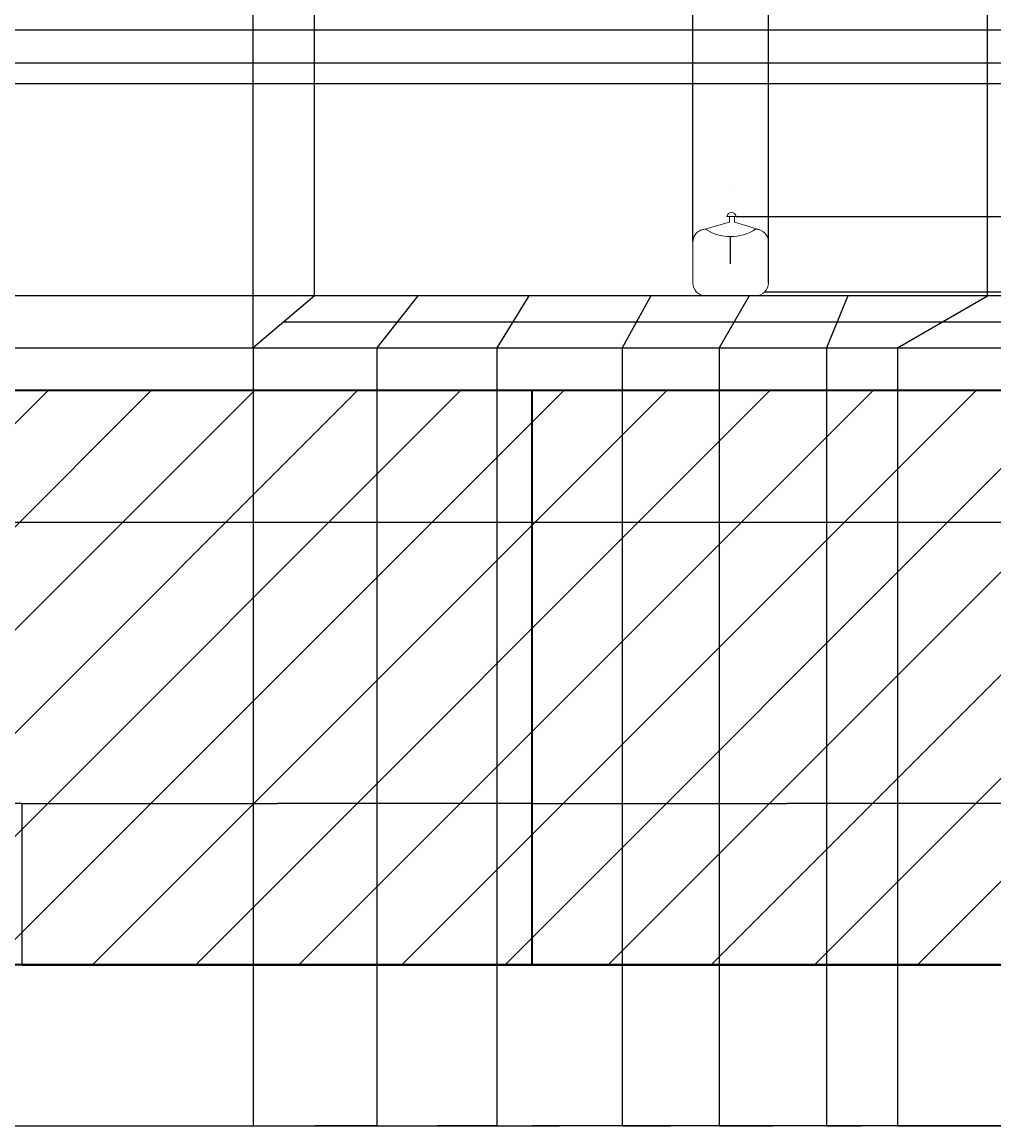
# Model space of a CAD drawing. Units: millimetres. Extents: x 2212 to 7718, y 1114 to 4219.
# Tile 2 of 5: x 4165 to 5689, y 1114 to 2844. Entities that reach past the tile are written whole.
import ezdxf

# ---------------------------------------------------------------- set-up
doc = ezdxf.new("R2010")
doc.units = ezdxf.units.MM
for name, color, linetype, lineweight in [('A-ANNO-DIMS', 2, 'Continuous', 18), ('A-ELEV-PATT', 8, 'Continuous', 13), ('A-EQPM', 4, 'Continuous', 25), ('A-FURN', 7, 'Continuous', 35), ('A-FURN-ACCS', 8, 'Continuous', 18), ('A-FURN-CTOP', 6, 'Continuous', 25)]:
    doc.layers.add(name, color=color, linetype=linetype, lineweight=lineweight)
doc.styles.get("Standard").update_dxf_attribs({"font": 'arial.ttf'})
doc.dimstyles.get("Standard").update_dxf_attribs({"dimtxt": 0.18, "dimasz": 0.18, "dimexe": 0.18, "dimexo": 0.0625, "dimgap": 0.09, "dimtad": 0, "dimtih": 1, "dimtoh": 1, "dimdec": 4, "dimzin": 0, "dimdsep": 46, "dimtxsty": 'Standard', "dimcen": 0.09, "dimadec": 0, "dimazin": 0, "dimtfac": 1, "dimtdec": 4, "dimtofl": 0, "dimtmove": 0, "dimatfit": 3, "dimfxl": 1, "dimtolj": 1, "dimtzin": 0, "dimarcsym": 0})

# ---------------------------------------------------------------- blocks, each defined once
blk = doc.blocks.new('*D14')
at = {"layer": 'A-ANNO-DIMS', "color": 0, "lineweight": -2, "transparency": 16777216}
for p, q in [((3365.1, 1366.2), (3365.1, 1618.9)), ((3365.3, 1618.7), (3764.9, 1618.7)), ((4165, 1618.7), (3765.4, 1618.7)), ((4165.1, 1366.2), (4165.1, 1618.9))]:
    blk.add_line(p, q, dxfattribs=at)
at = {"layer": 'A-ANNO-DIMS', "color": 0, "transparency": 16777216}
for points in [[(3365.3, 1618.7), (3365.3, 1618.7), (3365.1, 1618.7)], [(4165, 1618.7), (4165, 1618.7), (4165.1, 1618.7)]]:
    blk.add_solid(points, dxfattribs=at)
at = {"layer": 'Defpoints', "color": 0, "transparency": 16777216}
for p in [(4165.1, 1618.7), (3365.1, 1366.2), (4165.1, 1366.2)]:
    blk.add_point(p, dxfattribs=at)
at = {"layer": 'A-ANNO-DIMS', "color": 0, "transparency": 16777216, "insert": (3765.1, 1618.7), "char_height": 0.18, "attachment_point": 5}
blk.add_mtext('\\A1;800', dxfattribs=at)
blk = doc.blocks.new('*D15')
at = {"layer": 'A-ANNO-DIMS', "color": 0, "lineweight": -2, "transparency": 16777216}
for p, q in [((4165.1, 1366.2), (4165.1, 1618.9)), ((4165.3, 1618.7), (4564.9, 1618.7)), ((4965, 1618.7), (4565.4, 1618.7)), ((4965.1, 1366.2), (4965.1, 1618.9))]:
    blk.add_line(p, q, dxfattribs=at)
at = {"layer": 'A-ANNO-DIMS', "color": 0, "transparency": 16777216}
for points in [[(4165.3, 1618.7), (4165.3, 1618.7), (4165.1, 1618.7)], [(4965, 1618.7), (4965, 1618.7), (4965.1, 1618.7)]]:
    blk.add_solid(points, dxfattribs=at)
at = {"layer": 'Defpoints', "color": 0, "transparency": 16777216}
for p in [(4965.1, 1618.7), (4165.1, 1366.2), (4965.1, 1366.2)]:
    blk.add_point(p, dxfattribs=at)
at = {"layer": 'A-ANNO-DIMS', "color": 0, "transparency": 16777216, "insert": (4565.1, 1618.7), "char_height": 0.18, "attachment_point": 5}
blk.add_mtext('\\A1;800', dxfattribs=at)
blk = doc.blocks.new('*D16')
at = {"layer": 'A-ANNO-DIMS', "color": 0, "lineweight": -2, "transparency": 16777216}
for p, q in [((4965.1, 1366.2), (4965.1, 1618.9)), ((4965.3, 1618.7), (5364.9, 1618.7)), ((5765, 1618.7), (5365.4, 1618.7)), ((5765.1, 1366.2), (5765.1, 1618.9))]:
    blk.add_line(p, q, dxfattribs=at)
at = {"layer": 'A-ANNO-DIMS', "color": 0, "transparency": 16777216}
for points in [[(4965.3, 1618.7), (4965.3, 1618.7), (4965.1, 1618.7)], [(5765, 1618.7), (5765, 1618.7), (5765.1, 1618.7)]]:
    blk.add_solid(points, dxfattribs=at)
at = {"layer": 'Defpoints', "color": 0, "transparency": 16777216}
for p in [(5765.1, 1618.7), (4965.1, 1366.2), (5765.1, 1366.2)]:
    blk.add_point(p, dxfattribs=at)
at = {"layer": 'A-ANNO-DIMS', "color": 0, "transparency": 16777216, "insert": (5365.1, 1618.7), "char_height": 0.18, "attachment_point": 5}
blk.add_mtext('\\A1;800', dxfattribs=at)
blk = doc.blocks.new('*D18')
at = {"layer": 'A-ANNO-DIMS', "color": 0, "lineweight": -2, "transparency": 16777216}
for p, q in [((2465.1, 1366.1), (2465.1, 1113.5)), ((7465.1, 1366.1), (7465.1, 1113.5)), ((2465.3, 1113.7), (4964.8, 1113.7)), ((7465, 1113.7), (4965.5, 1113.7))]:
    blk.add_line(p, q, dxfattribs=at)
at = {"layer": 'A-ANNO-DIMS', "color": 0, "transparency": 16777216}
for points in [[(2465.3, 1113.7), (2465.3, 1113.7), (2465.1, 1113.7)], [(7465, 1113.7), (7465, 1113.7), (7465.1, 1113.7)]]:
    blk.add_solid(points, dxfattribs=at)
at = {"layer": 'Defpoints', "color": 0, "transparency": 16777216}
for p in [(2465.1, 1366.2), (7465.1, 1366.2), (7465.1, 1113.7)]:
    blk.add_point(p, dxfattribs=at)
at = {"layer": 'A-ANNO-DIMS', "color": 0, "transparency": 16777216, "insert": (4965.1, 1113.7), "char_height": 0.18, "attachment_point": 5}
blk.add_mtext('\\A1;5000', dxfattribs=at)
blk = doc.blocks.new('*D27')
at = {"layer": 'A-ANNO-DIMS', "color": 0, "lineweight": -2, "transparency": 16777216}
for p, q in [((5865.1, 2746.8), (2212.5, 2746.8)), ((2212.6, 2746.6), (2212.6, 2403.4)), ((2212.6, 2059.8), (2212.6, 2403)), ((5865.1, 2059.6), (2212.5, 2059.6))]:
    blk.add_line(p, q, dxfattribs=at)
at = {"layer": 'A-ANNO-DIMS', "color": 0, "transparency": 16777216}
for points in [[(2212.6, 2746.6), (2212.7, 2746.6), (2212.6, 2746.8)], [(2212.6, 2059.8), (2212.7, 2059.8), (2212.6, 2059.6)]]:
    blk.add_solid(points, dxfattribs=at)
at = {"layer": 'Defpoints', "color": 0, "transparency": 16777216}
for p in [(2212.6, 2746.8), (5865.1, 2746.8), (5865.1, 2059.6)]:
    blk.add_point(p, dxfattribs=at)
at = {"layer": 'A-ANNO-DIMS', "color": 0, "transparency": 16777216, "insert": (2212.6, 2403.2), "char_height": 0.18, "attachment_point": 5}
blk.add_mtext('\\A1;687.2', dxfattribs=at)
blk = doc.blocks.new('*D28')
at = {"layer": 'A-ANNO-DIMS', "color": 0, "lineweight": -2, "transparency": 16777216}
for p, q in [((5865.1, 2856.7), (2212.5, 2856.7)), ((2212.6, 2856.6), (2212.6, 2802)), ((2212.6, 2747), (2212.6, 2801.6)), ((5865.1, 2746.8), (2212.5, 2746.8))]:
    blk.add_line(p, q, dxfattribs=at)
at = {"layer": 'A-ANNO-DIMS', "color": 0, "transparency": 16777216}
for points in [[(2212.6, 2856.6), (2212.7, 2856.6), (2212.6, 2856.7)], [(2212.6, 2747), (2212.7, 2747), (2212.6, 2746.8)]]:
    blk.add_solid(points, dxfattribs=at)
at = {"layer": 'Defpoints', "color": 0, "transparency": 16777216}
for p in [(2212.6, 2856.7), (5865.1, 2856.7), (5865.1, 2746.8)]:
    blk.add_point(p, dxfattribs=at)
at = {"layer": 'A-ANNO-DIMS', "color": 0, "transparency": 16777216, "insert": (2212.6, 2801.8), "char_height": 0.18, "attachment_point": 5}
blk.add_mtext('\\A1;109.95', dxfattribs=at)
blk = doc.blocks.new('*D44')
at = {"layer": 'A-ANNO-DIMS', "color": 0, "lineweight": -2, "transparency": 16777216}
for p, q in [((6023.8, 2830.9), (2212.5, 2830.9)), ((2212.6, 2830.7), (2212.6, 2805.3)), ((2212.6, 2779.5), (2212.6, 2804.9)), ((6023.8, 2779.3), (2212.5, 2779.3))]:
    blk.add_line(p, q, dxfattribs=at)
at = {"layer": 'A-ANNO-DIMS', "color": 0, "transparency": 16777216}
for points in [[(2212.6, 2830.7), (2212.7, 2830.7), (2212.6, 2830.9)], [(2212.6, 2779.5), (2212.7, 2779.5), (2212.6, 2779.3)]]:
    blk.add_solid(points, dxfattribs=at)
at = {"layer": 'Defpoints', "color": 0, "transparency": 16777216}
for p in [(2212.6, 2830.9), (6023.9, 2830.9), (6023.9, 2779.3)]:
    blk.add_point(p, dxfattribs=at)
at = {"layer": 'A-ANNO-DIMS', "color": 0, "transparency": 16777216, "insert": (2212.6, 2805.1), "char_height": 0.18, "attachment_point": 5}
blk.add_mtext('\\A1;51.58', dxfattribs=at)
blk = doc.blocks.new('*D56')
at = {"layer": 'A-ANNO-DIMS', "color": 0, "lineweight": -2, "transparency": 16777216}
for p, q in [((5275.9, 2579.1), (5276.1, 2579.1)), ((5276, 2579.1), (5276, 2579.2)), ((5276, 2464.6), (5276, 2507.4)), ((5275.8, 2464.6), (5276, 2464.6))]:
    blk.add_line(p, q, dxfattribs=at)
at = {"layer": 'A-ANNO-DIMS', "color": 0, "transparency": 16777216}
blk.add_solid([(5276, 2507.4), (5276.1, 2507.4), (5276, 2507.5)], dxfattribs=at)
at = {"layer": 'Defpoints', "color": 0, "transparency": 16777216}
for p in [(5276, 2579.1), (5276, 2507.5)]:
    blk.add_point(p, dxfattribs=at)
at = {"layer": 'A-ANNO-DIMS', "color": 0, "transparency": 16777216, "insert": (5275.4, 2464.6), "char_height": 0.18, "attachment_point": 5}
blk.add_mtext('\\A1;R71.61', dxfattribs=at)
blk = doc.blocks.new('*D62')
at = {"layer": 'A-ANNO-DIMS', "color": 0, "lineweight": -2, "transparency": 16777216}
for p, q in [((5537.5, 2333.3), (5537.5, 1113.5)), ((5865.1, 2333.3), (5865.1, 1113.5)), ((5537.7, 1113.7), (5700.8, 1113.7)), ((5865, 1113.7), (5701.8, 1113.7))]:
    blk.add_line(p, q, dxfattribs=at)
at = {"layer": 'A-ANNO-DIMS', "color": 0, "transparency": 16777216}
for points in [[(5537.7, 1113.7), (5537.7, 1113.7), (5537.5, 1113.7)], [(5865, 1113.7), (5865, 1113.7), (5865.1, 1113.7)]]:
    blk.add_solid(points, dxfattribs=at)
at = {"layer": 'Defpoints', "color": 0, "transparency": 16777216}
for p in [(5537.5, 2333.4), (5865.1, 2333.4), (5865.1, 1113.7)]:
    blk.add_point(p, dxfattribs=at)
at = {"layer": 'A-ANNO-DIMS', "color": 0, "transparency": 16777216, "insert": (5701.3, 1113.7), "char_height": 0.18, "attachment_point": 5}
blk.add_mtext('\\A1;327.66', dxfattribs=at)
blk = doc.blocks.new('*D63')
at = {"layer": 'A-ANNO-DIMS', "color": 0, "lineweight": -2, "transparency": 16777216}
for p, q in [((4527.5, 2333.3), (4527.5, 1113.5)), ((4721.2, 2333.3), (4721.2, 1113.5)), ((4527.7, 1113.7), (4623.9, 1113.7)), ((4721.1, 1113.7), (4624.8, 1113.7))]:
    blk.add_line(p, q, dxfattribs=at)
at = {"layer": 'A-ANNO-DIMS', "color": 0, "transparency": 16777216}
for points in [[(4527.7, 1113.7), (4527.7, 1113.7), (4527.5, 1113.7)], [(4721.1, 1113.7), (4721.1, 1113.7), (4721.2, 1113.7)]]:
    blk.add_solid(points, dxfattribs=at)
at = {"layer": 'Defpoints', "color": 0, "transparency": 16777216}
for p in [(4527.5, 2333.4), (4721.2, 2333.4), (4721.2, 1113.7)]:
    blk.add_point(p, dxfattribs=at)
at = {"layer": 'A-ANNO-DIMS', "color": 0, "transparency": 16777216, "insert": (4624.4, 1113.7), "char_height": 0.18, "attachment_point": 5}
blk.add_mtext('\\A1;193.73', dxfattribs=at)
blk = doc.blocks.new('*D64')
at = {"layer": 'A-ANNO-DIMS', "color": 0, "lineweight": -2, "transparency": 16777216}
for p, q in [((4721.2, 2333.3), (4721.2, 1113.5)), ((4909.6, 2333.3), (4909.6, 1113.5)), ((4721.4, 1113.7), (4814.9, 1113.7)), ((4909.4, 1113.7), (4815.9, 1113.7))]:
    blk.add_line(p, q, dxfattribs=at)
at = {"layer": 'A-ANNO-DIMS', "color": 0, "transparency": 16777216}
for points in [[(4721.4, 1113.7), (4721.4, 1113.7), (4721.2, 1113.7)], [(4909.4, 1113.7), (4909.4, 1113.7), (4909.6, 1113.7)]]:
    blk.add_solid(points, dxfattribs=at)
at = {"layer": 'Defpoints', "color": 0, "transparency": 16777216}
for p in [(4721.2, 2333.4), (4909.6, 2333.4), (4909.6, 1113.7)]:
    blk.add_point(p, dxfattribs=at)
at = {"layer": 'A-ANNO-DIMS', "color": 0, "transparency": 16777216, "insert": (4815.4, 1113.7), "char_height": 0.18, "attachment_point": 5}
blk.add_mtext('\\A1;188.32', dxfattribs=at)
blk = doc.blocks.new('*D65')
at = {"layer": 'A-ANNO-DIMS', "color": 0, "lineweight": -2, "transparency": 16777216}
for p, q in [((4909.6, 2333.3), (4909.6, 1113.5)), ((5106.1, 2333.3), (5106.1, 1113.5)), ((4909.7, 1113.7), (5007.4, 1113.7)), ((5105.9, 1113.7), (5008.3, 1113.7))]:
    blk.add_line(p, q, dxfattribs=at)
at = {"layer": 'A-ANNO-DIMS', "color": 0, "transparency": 16777216}
for points in [[(4909.7, 1113.7), (4909.7, 1113.7), (4909.6, 1113.7)], [(5105.9, 1113.7), (5105.9, 1113.7), (5106.1, 1113.7)]]:
    blk.add_solid(points, dxfattribs=at)
at = {"layer": 'Defpoints', "color": 0, "transparency": 16777216}
for p in [(4909.6, 2333.4), (5106.1, 2333.4), (5106.1, 1113.7)]:
    blk.add_point(p, dxfattribs=at)
at = {"layer": 'A-ANNO-DIMS', "color": 0, "transparency": 16777216, "insert": (5007.8, 1113.7), "char_height": 0.18, "attachment_point": 5}
blk.add_mtext('\\A1;196.54', dxfattribs=at)
blk = doc.blocks.new('*D66')
at = {"layer": 'A-ANNO-DIMS', "color": 0, "lineweight": -2, "transparency": 16777216}
for p, q in [((5106.1, 2333.3), (5106.1, 1113.5)), ((5257.9, 2333.3), (5257.9, 1113.5)), ((5106.3, 1113.7), (5181.6, 1113.7)), ((5257.7, 1113.7), (5182.5, 1113.7))]:
    blk.add_line(p, q, dxfattribs=at)
at = {"layer": 'A-ANNO-DIMS', "color": 0, "transparency": 16777216}
for points in [[(5106.3, 1113.7), (5106.3, 1113.7), (5106.1, 1113.7)], [(5257.7, 1113.7), (5257.7, 1113.7), (5257.9, 1113.7)]]:
    blk.add_solid(points, dxfattribs=at)
at = {"layer": 'Defpoints', "color": 0, "transparency": 16777216}
for p in [(5106.1, 2333.4), (5257.9, 2333.4), (5257.9, 1113.7)]:
    blk.add_point(p, dxfattribs=at)
at = {"layer": 'A-ANNO-DIMS', "color": 0, "transparency": 16777216, "insert": (5182, 1113.7), "char_height": 0.18, "attachment_point": 5}
blk.add_mtext('\\A1;151.80', dxfattribs=at)
blk = doc.blocks.new('*D67')
at = {"layer": 'A-ANNO-DIMS', "color": 0, "lineweight": -2, "transparency": 16777216}
for p, q in [((5257.9, 2333.3), (5257.9, 1113.5)), ((5426.3, 2333.3), (5426.3, 1113.5)), ((5258.1, 1113.7), (5341.6, 1113.7)), ((5426.1, 1113.7), (5342.5, 1113.7))]:
    blk.add_line(p, q, dxfattribs=at)
at = {"layer": 'A-ANNO-DIMS', "color": 0, "transparency": 16777216}
for points in [[(5258.1, 1113.7), (5258.1, 1113.7), (5257.9, 1113.7)], [(5426.1, 1113.7), (5426.1, 1113.7), (5426.3, 1113.7)]]:
    blk.add_solid(points, dxfattribs=at)
at = {"layer": 'Defpoints', "color": 0, "transparency": 16777216}
for p in [(5257.9, 2333.4), (5426.3, 2333.4), (5426.3, 1113.7)]:
    blk.add_point(p, dxfattribs=at)
at = {"layer": 'A-ANNO-DIMS', "color": 0, "transparency": 16777216, "insert": (5342.1, 1113.7), "char_height": 0.18, "attachment_point": 5}
blk.add_mtext('\\A1;168.35', dxfattribs=at)
blk = doc.blocks.new('*D68')
at = {"layer": 'A-ANNO-DIMS', "color": 0, "lineweight": -2, "transparency": 16777216}
for p, q in [((5426.3, 2333.3), (5426.3, 1113.5)), ((5537.5, 2333.3), (5537.5, 1113.5)), ((5426.4, 1113.7), (5481.4, 1113.7)), ((5537.3, 1113.7), (5482.3, 1113.7))]:
    blk.add_line(p, q, dxfattribs=at)
at = {"layer": 'A-ANNO-DIMS', "color": 0, "transparency": 16777216}
for points in [[(5426.4, 1113.7), (5426.4, 1113.7), (5426.3, 1113.7)], [(5537.3, 1113.7), (5537.3, 1113.7), (5537.5, 1113.7)]]:
    blk.add_solid(points, dxfattribs=at)
at = {"layer": 'Defpoints', "color": 0, "transparency": 16777216}
for p in [(5426.3, 2333.4), (5537.5, 2333.4), (5537.5, 1113.7)]:
    blk.add_point(p, dxfattribs=at)
at = {"layer": 'A-ANNO-DIMS', "color": 0, "transparency": 16777216, "insert": (5481.9, 1113.7), "char_height": 0.18, "attachment_point": 5}
blk.add_mtext('\\A1;111.22', dxfattribs=at)
blk = doc.blocks.new('*D69')
at = {"layer": 'A-ANNO-DIMS', "color": 0, "lineweight": -2, "transparency": 16777216}
for p, q in [((4623.4, 2414.9), (4623.4, 4218.9)), ((4623.6, 4218.7), (5150.6, 4218.7)), ((5678.7, 4218.7), (5151.6, 4218.7)), ((5678.9, 2414.9), (5678.9, 4218.9))]:
    blk.add_line(p, q, dxfattribs=at)
at = {"layer": 'A-ANNO-DIMS', "color": 0, "transparency": 16777216}
for points in [[(4623.6, 4218.7), (4623.6, 4218.7), (4623.4, 4218.7)], [(5678.7, 4218.7), (5678.7, 4218.7), (5678.9, 4218.7)]]:
    blk.add_solid(points, dxfattribs=at)
at = {"layer": 'Defpoints', "color": 0, "transparency": 16777216}
for p in [(5678.9, 4218.7), (4623.4, 2414.8), (5678.9, 2414.8)]:
    blk.add_point(p, dxfattribs=at)
at = {"layer": 'A-ANNO-DIMS', "color": 0, "transparency": 16777216, "insert": (5151.1, 4218.7), "char_height": 0.18, "attachment_point": 5}
blk.add_mtext('\\A1;1055.48', dxfattribs=at)
blk = doc.blocks.new('*D70')
at = {"layer": 'A-ANNO-DIMS', "color": 0, "lineweight": -2, "transparency": 16777216}
for p, q in [((4527.5, 2333.4), (4527.5, 4218.9)), ((4527.7, 4218.7), (4575.1, 4218.7)), ((4623.2, 4218.7), (4575.8, 4218.7)), ((4623.4, 2414.9), (4623.4, 4218.9))]:
    blk.add_line(p, q, dxfattribs=at)
at = {"layer": 'A-ANNO-DIMS', "color": 0, "transparency": 16777216}
for points in [[(4527.7, 4218.7), (4527.7, 4218.7), (4527.5, 4218.7)], [(4623.2, 4218.7), (4623.2, 4218.7), (4623.4, 4218.7)]]:
    blk.add_solid(points, dxfattribs=at)
at = {"layer": 'Defpoints', "color": 0, "transparency": 16777216}
for p in [(4623.4, 4218.7), (4623.4, 2414.8), (4527.5, 2333.4)]:
    blk.add_point(p, dxfattribs=at)
at = {"layer": 'A-ANNO-DIMS', "color": 0, "transparency": 16777216, "insert": (4575.4, 4218.7), "char_height": 0.18, "attachment_point": 5}
blk.add_mtext('\\A1;95.87', dxfattribs=at)
blk = doc.blocks.new('*D71')
at = {"layer": 'A-ANNO-DIMS', "color": 0, "lineweight": -2, "transparency": 16777216}
for p, q in [((5608.2, 2374.1), (7717.8, 2374.1)), ((7717.6, 2373.9), (7717.6, 2353.9)), ((7717.6, 2333.5), (7717.6, 2353.5)), ((5537.5, 2333.4), (7717.8, 2333.4))]:
    blk.add_line(p, q, dxfattribs=at)
at = {"layer": 'A-ANNO-DIMS', "color": 0, "transparency": 16777216}
for points in [[(7717.6, 2373.9), (7717.7, 2373.9), (7717.6, 2374.1)], [(7717.6, 2333.5), (7717.7, 2333.5), (7717.6, 2333.4)]]:
    blk.add_solid(points, dxfattribs=at)
at = {"layer": 'Defpoints', "color": 0, "transparency": 16777216}
for p in [(5608.2, 2374.1), (7717.6, 2374.1), (5537.5, 2333.4)]:
    blk.add_point(p, dxfattribs=at)
at = {"layer": 'A-ANNO-DIMS', "color": 0, "transparency": 16777216, "insert": (7717.6, 2353.7), "char_height": 0.18, "attachment_point": 5}
blk.add_mtext('\\A1;40.726', dxfattribs=at)
blk = doc.blocks.new('*D72')
at = {"layer": 'A-ANNO-DIMS', "color": 0, "lineweight": -2, "transparency": 16777216}
for p, q in [((5216.8, 2499.3), (5216.8, 4218.9)), ((5217, 4218.7), (5275.6, 4218.7)), ((5335, 4218.7), (5276.5, 4218.7)), ((5335.2, 2499.3), (5335.2, 4218.9))]:
    blk.add_line(p, q, dxfattribs=at)
at = {"layer": 'A-ANNO-DIMS', "color": 0, "transparency": 16777216}
for points in [[(5217, 4218.7), (5217, 4218.7), (5216.8, 4218.7)], [(5335, 4218.7), (5335, 4218.7), (5335.2, 4218.7)]]:
    blk.add_solid(points, dxfattribs=at)
at = {"layer": 'Defpoints', "color": 0, "transparency": 16777216}
for p in [(5335.2, 4218.7), (5216.8, 2499.2), (5335.2, 2499.2)]:
    blk.add_point(p, dxfattribs=at)
at = {"layer": 'A-ANNO-DIMS', "color": 0, "transparency": 16777216, "insert": (5276, 4218.7), "char_height": 0.18, "attachment_point": 5}
blk.add_mtext('\\A1;118.35', dxfattribs=at)
blk = doc.blocks.new('*D73')
at = {"layer": 'A-ANNO-DIMS', "color": 0, "lineweight": -2, "transparency": 16777216}
for p, q in [((5284.8, 2539.3), (7717.8, 2539.3)), ((7717.6, 2539.1), (7717.6, 2480.2)), ((7717.6, 2420.9), (7717.6, 2479.8)), ((5329.4, 2420.7), (7717.8, 2420.7))]:
    blk.add_line(p, q, dxfattribs=at)
at = {"layer": 'A-ANNO-DIMS', "color": 0, "transparency": 16777216}
for points in [[(7717.6, 2539.1), (7717.7, 2539.1), (7717.6, 2539.3)], [(7717.6, 2420.9), (7717.7, 2420.9), (7717.6, 2420.7)]]:
    blk.add_solid(points, dxfattribs=at)
at = {"layer": 'Defpoints', "color": 0, "transparency": 16777216}
for p in [(5284.8, 2539.3), (7717.6, 2539.3), (5329.3, 2420.7)]:
    blk.add_point(p, dxfattribs=at)
at = {"layer": 'A-ANNO-DIMS', "color": 0, "transparency": 16777216, "insert": (7717.6, 2480), "char_height": 0.18, "attachment_point": 5}
blk.add_mtext('\\A1;118.60', dxfattribs=at)
blk = doc.blocks.new('*D74')
at = {"layer": 'A-ANNO-DIMS', "color": 0, "lineweight": -2, "transparency": 16777216}
for p, q in [((5335.2, 2434.9), (5335.2, 4218.9)), ((5335.4, 4218.7), (5599.7, 4218.7)), ((5865, 4218.7), (5600.6, 4218.7)), ((5865.1, 2414.9), (5865.1, 4218.9))]:
    blk.add_line(p, q, dxfattribs=at)
at = {"layer": 'A-ANNO-DIMS', "color": 0, "transparency": 16777216}
for points in [[(5335.4, 4218.7), (5335.4, 4218.7), (5335.2, 4218.7)], [(5865, 4218.7), (5865, 4218.7), (5865.1, 4218.7)]]:
    blk.add_solid(points, dxfattribs=at)
at = {"layer": 'Defpoints', "color": 0, "transparency": 16777216}
for p in [(5865.1, 4218.7), (5335.2, 2434.8), (5865.1, 2414.8)]:
    blk.add_point(p, dxfattribs=at)
at = {"layer": 'A-ANNO-DIMS', "color": 0, "transparency": 16777216, "insert": (5600.2, 4218.7), "char_height": 0.18, "attachment_point": 5}
blk.add_mtext('\\A1;529.94', dxfattribs=at)
blk = doc.blocks.new('*D75')
at = {"layer": 'A-ANNO-DIMS', "color": 0, "lineweight": -2, "transparency": 16777216}
for p, q in [((5275.9, 2579.1), (5276.1, 2579.1)), ((5276, 2579.1), (5276, 2579.2)), ((5276, 2464.6), (5276, 2507.4)), ((5275.8, 2464.6), (5276, 2464.6))]:
    blk.add_line(p, q, dxfattribs=at)
at = {"layer": 'A-ANNO-DIMS', "color": 0, "transparency": 16777216}
blk.add_solid([(5276, 2507.4), (5276.1, 2507.4), (5276, 2507.5)], dxfattribs=at)
at = {"layer": 'Defpoints', "color": 0, "transparency": 16777216}
for p in [(5276, 2579.1), (5276, 2507.5)]:
    blk.add_point(p, dxfattribs=at)
at = {"layer": 'A-ANNO-DIMS', "color": 0, "transparency": 16777216, "insert": (5275.4, 2464.6), "char_height": 0.18, "attachment_point": 5}
blk.add_mtext('\\A1;R71.61', dxfattribs=at)

msp = doc.modelspace()

# ---------------------------------------------------------------- hatches: boundary and pattern name
at = {"layer": 'A-ELEV-PATT'}
h = msp.add_hatch(dxfattribs=at)
h.set_pattern_fill('ANSI31', color=256, scale=36)
h.paths.add_polyline_path([(3153.454, 3966.1829), (2465.1412, 3966.1829), (2465.1412, 3121.3339), (3153.454, 3121.3339)])
h.paths.add_polyline_path([(3659.2976, 3966.1829), (3153.454, 3966.1829), (3153.454, 3121.3339), (3659.2976, 3121.3339)])
h.paths.add_polyline_path([(4165.1412, 3966.1829), (3659.2976, 3966.1829), (3659.2976, 3121.3339), (4165.1412, 3121.3339)])
h.paths.add_polyline_path([(3365.1412, 2266.3983), (2465.1412, 2266.3983), (2465.1412, 1366.1829), (3365.1412, 1366.1829)])
h.paths.add_polyline_path([(4165.1412, 2266.3983), (3365.1412, 2266.3983), (3365.1412, 1366.1829), (4165.1412, 1366.1829)])
h.paths.add_polyline_path([(4965.1412, 2266.3983), (4165.1412, 2266.3983), (4165.1412, 1366.1829), (4965.1412, 1366.1829)])
h.paths.add_polyline_path([(5765.1412, 2266.3983), (4965.1412, 2266.3983), (4965.1412, 1366.1829), (5765.1412, 1366.1829)])
h.paths.add_polyline_path([(6665.1412, 2059.6125), (5865.1412, 2059.6125), (5865.1412, 1366.1829), (6665.1412, 1366.1829)])
h.paths.add_polyline_path([(7465.1412, 2266.3983), (7065.1412, 2266.3983), (7065.1412, 1366.1829), (7465.1412, 1366.1829)])
h.paths.add_polyline_path([(7065.1412, 2266.3983), (6665.1412, 2266.3983), (6665.1412, 1366.1829), (7065.1412, 1366.1829)])
h.paths.add_polyline_path([(7465.1412, 3966.1829), (7065.1412, 3966.1829), (7065.1412, 2266.3983), (7465.1412, 2266.3983)])
h.paths.add_polyline_path([(7065.1412, 3966.1829), (6665.1412, 3966.1829), (6665.1412, 2266.3983), (7065.1412, 2266.3983)])
h.paths.add_polyline_path([(6665.1412, 3966.1829), (6027.7806, 3966.1829), (6027.7806, 3314.3715), (6665.1412, 3314.3715)])
h.paths.add_polyline_path([(5245.7331, 3966.1829), (4821.5849, 3966.1829), (4821.5849, 3216.3983), (4356.7186, 3216.3983), (4356.7186, 3121.3339), (5503.6152, 3121.3339), (5720.779, 3121.3339), (5720.779, 3216.3983), (5245.7331, 3216.3983)])

# ---------------------------------------------------------------- linework, layer by layer
at = {"layer": 'A-EQPM'}
for p, q in [((4623.3786, 2414.8193), (4527.5091, 2333.3682)), ((5678.8596, 2414.8193), (4623.3786, 2414.8193)), ((4785.623, 2414.8193), (4721.2407, 2333.3682)), ((4959.7855, 2414.8193), (4909.5655, 2333.3682)), ((5151.1191, 2414.8193), (5106.1086, 2333.3682)), ((5305.2764, 2414.8193), (5257.9099, 2333.3682)), ((5459.9311, 2414.8193), (5426.2609, 2333.3682)), ((5537.4832, 2333.3682), (5678.8596, 2414.8193)), ((4575.4439, 2374.0937), (5608.1714, 2374.0937)), ((4527.5091, 2333.3682), (5537.4832, 2333.3682))]:
    msp.add_line(p, q, dxfattribs=at)
at = {"layer": 'A-FURN'}
for p, q in [((5765.1412, 2266.3983), (2465.1412, 2266.3983)), ((4965.1412, 1366.1829), (4965.1412, 2266.3983)), ((5865.1412, 1366.1829), (2465.1412, 1366.1829)), ((4165.1412, 1366.1829), (4965.1412, 1366.1829)), ((4965.1412, 1366.1829), (5765.1412, 1366.1829))]:
    msp.add_line(p, q, dxfattribs=at)
at = {"layer": 'A-FURN-ACCS'}
for p, q in [((5274.027, 2529.981), (5228.0995, 2517.188)), ((5274.027, 2539.2808), (5270.2392, 2539.2808)), ((5270.2392, 2539.2808), (5284.7847, 2539.2808)), ((5274.027, 2539.2808), (5274.027, 2529.981)), ((5281.9041, 2539.2808), (5281.9041, 2529.981)), ((5281.9041, 2529.981), (5321.765, 2518.224)), ((5321.765, 2518.224), (5321.7023, 2518.113))]:
    msp.add_line(p, q, dxfattribs=at)
msp.add_lwpolyline([(5315.1967, 2519.2007, -0.414213562), (5335.1967, 2499.2007), (5335.1967, 2434.8193, -0.414213562), (5315.1967, 2414.8193), (5236.8434, 2414.8193, -0.414213562), (5216.8434, 2434.8193), (5216.8434, 2499.2007, -0.414213562), (5236.8434, 2519.2007)], format="xyb", dxfattribs=at)
for centre, radius, start, end in [((5277.512, 2537.7961), 7.4228, 11.5382357, 168.4617643), ((5276.0201, 2579.1484), 71.6138, 236.8348401, 303.1651599)]:
    msp.add_arc(centre, radius, start, end, dxfattribs=at)
at = {"layer": 'A-FURN-CTOP'}
for p, q in [((5865.1412, 2414.8193), (2465.1412, 2414.8193)), ((2465.1412, 2333.3682), (5865.1412, 2333.3682))]:
    msp.add_line(p, q, dxfattribs=at)

# ---------------------------------------------------------------- dimensions: what is measured, and where the dimension line sits
at = {"layer": 'A-ANNO-DIMS'}
for base, p1, p2, override, picture, middle in [((4623.3786, 4218.6829), (4527.5091, 2333.3682), (4623.3786, 2414.8193), {"dimdec": 2, "dimlfac": 1, "dimrnd": 0, "dimzin": 0, "dimdsep": 46, "dimlunit": 2}, '*D70', (4575.4438, 4218.6829)), ((5678.8596, 4218.6829), (4623.3786, 2414.8193), (5678.8596, 2414.8193), {"dimdec": 2, "dimlfac": 1, "dimrnd": 0, "dimzin": 0, "dimdsep": 46, "dimlunit": 2}, '*D69', (5151.1191, 4218.6829)), ((5335.1967, 4218.6829), (5216.8434, 2499.2007), (5335.1967, 2499.2007), {"dimdec": 2, "dimlfac": 1, "dimrnd": 0, "dimzin": 0, "dimdsep": 46, "dimlunit": 2}, '*D72', (5276.0201, 4218.6829)), ((5865.1412, 4218.6829), (5335.1967, 2434.8193), (5865.1412, 2414.8193), {"dimdec": 2, "dimlfac": 1, "dimrnd": 0, "dimzin": 0, "dimdsep": 46, "dimlunit": 2}, '*D74', (5600.1689, 4218.6829)), ((4721.2407, 1113.6829), (4527.5091, 2333.3682), (4721.2407, 2333.3682), {"dimdec": 2, "dimlfac": 1, "dimrnd": 0, "dimzin": 0, "dimdsep": 46, "dimlunit": 2}, '*D63', (4624.3749, 1113.6829)), ((4909.5655, 1113.6829), (4721.2407, 2333.3682), (4909.5655, 2333.3682), {"dimdec": 2, "dimlfac": 1, "dimrnd": 0, "dimzin": 0, "dimdsep": 46, "dimlunit": 2}, '*D64', (4815.4031, 1113.6829)), ((5106.1086, 1113.6829), (4909.5655, 2333.3682), (5106.1086, 2333.3682), {"dimdec": 2, "dimlfac": 1, "dimrnd": 0, "dimzin": 0, "dimdsep": 46, "dimlunit": 2}, '*D65', (5007.8371, 1113.6829)), ((5257.9099, 1113.6829), (5106.1086, 2333.3682), (5257.9099, 2333.3682), {"dimdec": 2, "dimlfac": 1, "dimrnd": 0, "dimzin": 0, "dimdsep": 46, "dimlunit": 2}, '*D66', (5182.0093, 1113.6829)), ((5426.2609, 1113.6829), (5257.9099, 2333.3682), (5426.2609, 2333.3682), {"dimdec": 2, "dimlfac": 1, "dimrnd": 0, "dimzin": 0, "dimdsep": 46, "dimlunit": 2}, '*D67', (5342.0854, 1113.6829)), ((5537.4832, 1113.6829), (5426.2609, 2333.3682), (5537.4832, 2333.3682), {"dimdec": 2, "dimlfac": 1, "dimrnd": 0, "dimzin": 0, "dimdsep": 46, "dimlunit": 2}, '*D68', (5481.872, 1113.6829)), ((5865.1412, 1113.6829), (5537.4832, 2333.3682), (5865.1412, 2333.3682), {"dimdec": 2, "dimlfac": 1, "dimrnd": 0, "dimzin": 0, "dimdsep": 46, "dimlunit": 2}, '*D62', (5701.3122, 1113.6829)), ((4165.1412, 1618.6829), (3365.1412, 1366.1829), (4165.1412, 1366.1829), {"dimdec": 0, "dimlfac": 1, "dimrnd": 0, "dimzin": 0, "dimdsep": 46, "dimlunit": 2}, '*D14', (3765.1412, 1618.6829)), ((4965.1412, 1618.6829), (4165.1412, 1366.1829), (4965.1412, 1366.1829), {"dimdec": 0, "dimlfac": 1, "dimrnd": 0, "dimzin": 0, "dimdsep": 46, "dimlunit": 2}, '*D15', (4565.1412, 1618.6829)), ((5765.1412, 1618.6829), (4965.1412, 1366.1829), (5765.1412, 1366.1829), {"dimdec": 0, "dimlfac": 1, "dimrnd": 0, "dimzin": 0, "dimdsep": 46, "dimlunit": 2}, '*D16', (5365.1412, 1618.6829)), ((7465.1412, 1113.6829), (2465.1412, 1366.1829), (7465.1412, 1366.1829), {"dimdec": 0, "dimlfac": 1, "dimrnd": 0, "dimzin": 0, "dimdsep": 46, "dimlunit": 2}, '*D18', (4965.1412, 1113.6829))]:
    dim = msp.add_linear_dim(base=base, p1=p1, p2=p2, dimstyle='Standard', override=override, dxfattribs=at)
    dim.commit()
    dim.dimension.update_dxf_attribs({"geometry": picture, "text_midpoint": middle})
for base, p1, p2, override, picture, middle in [((2212.6412, 2856.7409), (5865.1412, 2746.7954), (5865.1412, 2856.7409), {"dimdec": 2, "dimlfac": 1, "dimrnd": 0, "dimzin": 0, "dimdsep": 46, "dimlunit": 2}, '*D28', (2212.6412, 2801.7682)), ((2212.6412, 2830.8799), (6023.8866, 2779.2966), (6023.8866, 2830.8799), {"dimdec": 2, "dimlfac": 1, "dimrnd": 0, "dimzin": 0, "dimdsep": 46, "dimlunit": 2}, '*D44', (2212.6412, 2805.0882)), ((2212.6412, 2746.7954), (5865.1412, 2059.6125), (5865.1412, 2746.7954), {"dimdec": 1, "dimlfac": 1, "dimrnd": 0, "dimzin": 0, "dimdsep": 46, "dimlunit": 2}, '*D27', (2212.6412, 2403.204)), ((7717.6412, 2539.2808), (5329.3388, 2420.6771), (5284.7847, 2539.2808), {"dimdec": 2, "dimlfac": 1, "dimrnd": 0, "dimzin": 0, "dimdsep": 46, "dimlunit": 2}, '*D73', (7717.6412, 2479.979)), ((7717.64116, 2374.09375), (5537.48322, 2333.36822), (5608.17143, 2374.09375), {"dimdec": 3, "dimlfac": 1, "dimrnd": 0, "dimzin": 0, "dimdsep": 46, "dimlunit": 2}, '*D71', (7717.64116, 2353.73098))]:
    dim = msp.add_linear_dim(base=base, p1=p1, p2=p2, angle=90, dimstyle='Standard', override=override, dxfattribs=at)
    dim.commit()
    dim.dimension.update_dxf_attribs({"geometry": picture, "text_midpoint": middle})
for picture in ['*D56', '*D75']:
    dim = msp.add_radius_dim(center=(5276.0201, 2579.1484), mpoint=(5276.02, 2507.5346), dimstyle='Standard', override={"dimdec": 2, "dimlfac": 1, "dimrnd": 0, "dimzin": 0, "dimdsep": 46, "dimlunit": 2}, dxfattribs=at)
    dim.commit()
    dim.dimension.update_dxf_attribs({"geometry": picture, "text_midpoint": (5275.3775, 2464.5663), "dimtype": 164})

doc.saveas('drawing.dxf')
